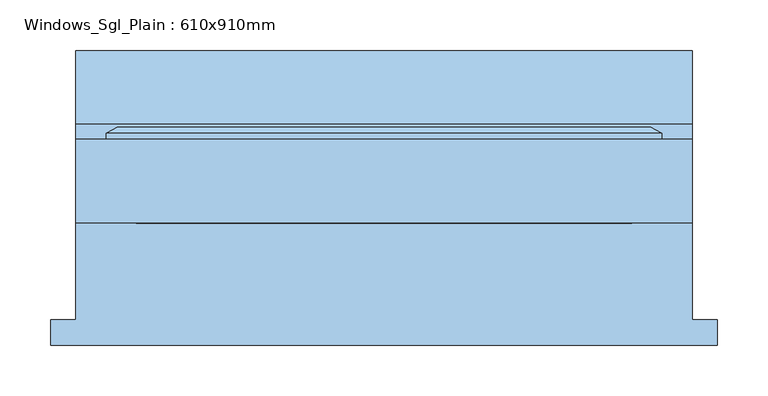
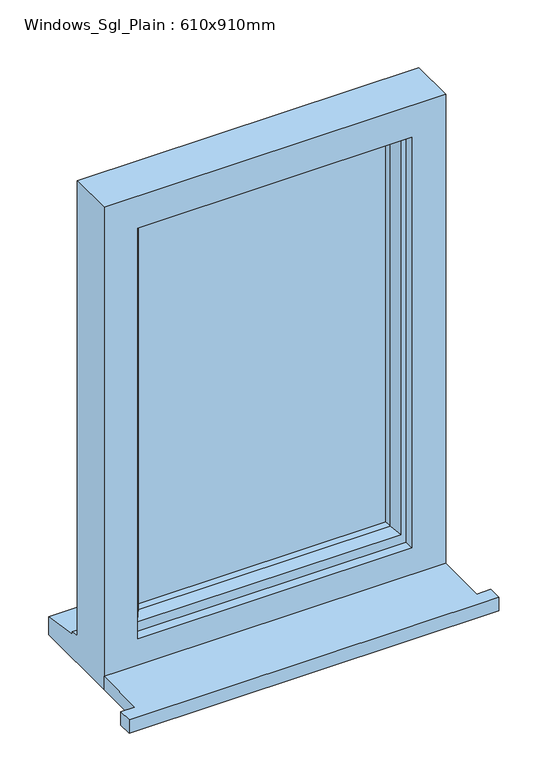
"""IFC4 building model written with IfcOpenShell, lengths in millimetres: window geometry, Windows_Sgl_Plain : 610x910mm."""

from ifc_helpers import new_model, si_unit, frame, origin, place, context, project, spatial, polyline, outline, extrude, faceted_brep, source, transform, mapped, element, save


def windows_sgl_plain_610x910mm_8d1346b0(model_context):
    return source(origin(), model_context, "Body", "SolidModel", [
        extrude(outline(polyline([(-329.8, -130.8434322), (-329.8, -105.8434322), (-304.8, -105.8434322), (-304.8, -10.2434322), (304.8, -10.2434322), (304.8, -105.8434322), (329.8, -105.8434322), (329.8, -130.8434322), (-329.8, -130.8434322)])), frame((0.0, 0.0, 1200.0), z_axis=(0.0, 0.0, 1.0), x_axis=(1.0, 0.0, 0.0)), (0.0, 0.0, 1.0), 25.0),
        faceted_brep([(-304.8, -10.2434322, 1200.0), (304.8, -10.2434322, 1200.0), (304.8, -10.2434322, 2110.0), (-304.8, -10.2434322, 2110.0), (-244.8, -10.2434322, 2050.0), (244.8, -10.2434322, 2050.0), (244.8, -10.2434322, 1275.0), (-244.8, -10.2434322, 1275.0), (-304.8, 72.7565678, 2110.0), (-304.8, 72.7565678, 1251.0), (-304.8, 87.7565678, 1249.68767), (-304.8, 87.7565678, 1244.7449676), (-304.8, 160.2565678, 1233.8088847), (-304.8, 160.2565678, 1200.0), (304.8, 72.7565678, 2110.0), (304.8, 72.7565678, 1251.0), (-264.8, 72.7565678, 2070.0), (-264.8, 72.7565678, 1263.0), (264.8, 72.7565678, 1263.0), (264.8, 72.7565678, 2070.0), (-264.8, 7.7565678, 2070.0), (-264.8, 7.7565678, 1263.0), (264.8, 7.7565678, 2070.0), (264.8, 7.7565678, 1263.0), (-244.8, 7.7565678, 2050.0), (-244.8, 7.7565678, 1275.0), (244.8, 7.7565678, 1275.0), (244.8, 7.7565678, 2050.0), (304.8, 160.2565678, 1200.0), (304.8, 160.2565678, 1233.8088847), (304.8, 87.7565678, 1244.7449676), (304.8, 87.7565678, 1249.68767)], [[[0, 1, 2, 3], [4, 5, 6, 7]], [[0, 3, 8, 9, 10, 11, 12, 13]], [[9, 8, 14, 15], [16, 17, 18, 19]], [[17, 16, 20, 21]], [[20, 22, 23, 21], [24, 25, 26, 27]], [[24, 4, 7, 25]], [[3, 2, 14, 8]], [[16, 19, 22, 20]], [[5, 4, 24, 27]], [[15, 14, 2, 1, 28, 29, 30, 31]], [[19, 18, 23, 22]], [[5, 27, 26, 6]], [[28, 1, 0, 13]], [[29, 28, 13, 12]], [[30, 29, 12, 11]], [[31, 30, 11, 10]], [[15, 31, 10, 9]], [[21, 23, 18, 17]], [[7, 6, 26, 25]]]),
        extrude(outline(polyline([(234.8, 36.7565678), (-234.8, 36.7565678), (-234.8, 60.7565678), (234.8, 60.7565678), (234.8, 36.7565678)])), frame((0.0, 0.0, 1293.0), z_axis=(0.0, 0.0, 1.0), x_axis=(1.0, 0.0, 0.0)), (0.0, 0.0, 1.0), 747.0),
        faceted_brep([(-274.8, 72.7565678, 2080.0), (-274.8, 78.5300705, 2080.0), (-274.8, 78.5300705, 1253.0), (-274.8, 72.7565678, 1253.0), (-264.8, 7.7565678, 2070.0), (-264.8, 72.7565678, 2070.0), (-264.8, 72.7565678, 1263.0), (-264.8, 7.7565678, 1263.0), (-224.8, 22.2494677, 2030.0), (-234.9480377, 7.7565678, 2040.1480377), (-234.9480377, 7.7565678, 1292.8519623), (-224.8, 22.2494677, 1303.0), (-224.8, 36.7565678, 2030.0), (-224.8, 36.7565678, 1303.0), (-234.8, 60.7565678, 2040.0), (-234.8, 36.7565678, 2040.0), (-234.8, 36.7565678, 1293.0), (-234.8, 60.7565678, 1293.0), (-224.8, 78.5300705, 2030.0), (-224.8, 60.7565678, 2030.0), (-224.8, 60.7565678, 1303.0), (-224.8, 78.5300705, 1303.0), (-242.2457548, 84.3035732, 2047.4457548), (-242.2457548, 84.3035732, 1285.5542452), (-264.0153903, 84.3035732, 2069.2153903), (-264.0153903, 84.3035732, 1263.7846097), (274.8, 78.5300705, 1253.0), (274.8, 72.7565678, 1253.0), (264.8, 72.7565678, 1263.0), (264.8, 7.7565678, 1263.0), (234.9480377, 7.7565678, 1292.8519623), (224.8, 22.2494677, 1303.0), (224.8, 36.7565678, 1303.0), (234.8, 36.7565678, 1293.0), (234.8, 60.7565678, 1293.0), (224.8, 60.7565678, 1303.0), (224.8, 78.5300705, 1303.0), (242.2457548, 84.3035732, 1285.5542452), (264.0153903, 84.3035732, 1263.7846097), (274.8, 78.5300705, 2080.0), (274.8, 72.7565678, 2080.0), (264.8, 72.7565678, 2070.0), (264.8, 7.7565678, 2070.0), (234.9480377, 7.7565678, 2040.1480377), (224.8, 22.2494677, 2030.0), (224.8, 36.7565678, 2030.0), (234.8, 36.7565678, 2040.0), (234.8, 60.7565678, 2040.0), (224.8, 60.7565678, 2030.0), (224.8, 78.5300705, 2030.0), (242.2457548, 84.3035732, 2047.4457548), (264.0153903, 84.3035732, 2069.2153903)], [[[0, 1, 2, 3]], [[4, 5, 6, 7]], [[8, 9, 10, 11]], [[12, 8, 11, 13]], [[14, 15, 16, 17]], [[18, 19, 20, 21]], [[22, 18, 21, 23]], [[1, 24, 25, 2]], [[3, 2, 26, 27]], [[7, 6, 28, 29]], [[11, 10, 30, 31]], [[13, 11, 31, 32]], [[17, 16, 33, 34]], [[21, 20, 35, 36]], [[23, 21, 36, 37]], [[2, 25, 38, 26]], [[27, 26, 39, 40]], [[29, 28, 41, 42]], [[31, 30, 43, 44]], [[32, 31, 44, 45]], [[34, 33, 46, 47]], [[36, 35, 48, 49]], [[37, 36, 49, 50]], [[26, 38, 51, 39]], [[40, 39, 1, 0]], [[3, 27, 40, 0], [5, 41, 28, 6]], [[42, 41, 5, 4]], [[7, 29, 42, 4], [9, 43, 30, 10]], [[44, 43, 9, 8]], [[45, 44, 8, 12]], [[15, 46, 33, 16], [13, 32, 45, 12]], [[47, 46, 15, 14]], [[17, 34, 47, 14], [19, 48, 35, 20]], [[49, 48, 19, 18]], [[50, 49, 18, 22]], [[24, 51, 38, 25], [23, 37, 50, 22]], [[39, 51, 24, 1]]]),
    ])


if __name__ == "__main__":
    model = new_model("IFC4")
    model_context = context("Model", 3, world=origin())
    ifc_project = project(units=[si_unit("LENGTHUNIT", "METRE", prefix="MILLI")], contexts=[model_context])
    site = spatial("IfcSite", under=ifc_project)
    building = spatial("IfcBuilding", under=site)
    placement = place(None, origin())
    windows_sgl_plain_610x910mm_shape = windows_sgl_plain_610x910mm_8d1346b0(model_context)
    element("IfcWindow", 1, ObjectType="Windows_Sgl_Plain : 610x910mm", at=placement, inside=building, context=model_context, shape_type="MappedRepresentation", body=[
        mapped(windows_sgl_plain_610x910mm_shape, transform((0.0, 0.0, 0.0), x_axis=(1.0, 0.0, 0.0), y_axis=(0.0, 1.0, 0.0), z_axis=(0.0, 0.0, 1.0))),
    ])
    save(model, "model.ifc")

# Revit data of these elements
# Type "Windows_Sgl_Plain : 610x910mm"
#   Type Mark = "44"
#   Operation = "SinglePanel"
#   Construction Type Id = "SGL"
#   Manufacturer = "Revit"
#   Keynote = "L10"
#   Analytic Construction = "Large single-glazed windows"
#   Wrap Layers (Ext) from Ext = 0' - 4.03543"
#   Wrap Layers (Int) from Ext = 0' - 6.98819"
#   Window Board Projection = 0' - 0.98425"
#   Window Board Extension = 0' - 0.98425"
#   Visual Light Transmittance = 0.9
#   Solar Heat Gain Coefficient = 0.86
#   Rough Width = 2' - 0"
#   Rough Height = 2' - 11.82677"
#   Height = 2' - 11.82677"
#   Width = 2' - 0"
#   Heat Transfer Coefficient (U) = 5.5617 W/(m²·K)
#   Glazing Thickness = 0' - 0.94488"
#   FrameOffset - External = 0' - 1.9685"
#   Frame Depth = 0' - 2.55906"
#   Default Head Height = 6' - 11.07087"
#   Cill Depth = 0' - 3.44488"
#   Cavity Closer Width = 0' - 1.9685"
#   Cavity Closer Offset from Ext = 0' - 4.03543"
#   Cavity Closer Depth = 0' - 3.34646"
#   Define Thermal Properties by = 1
#   Vis - Cavity Closers = yes
#   Define Thermal Properties by = 1
#   Material Trim = Window Frame
#   Material Glass = Glass
#   Material Frame = Window Frame
#   Wall Closure = (empty or 0)
# Element 1 (IfcWindow, "Windows_Sgl_Plain : 610x910mm")
#   Materials on its faces: "Window Frame", "Glass"
# Materials
#   "Window Frame": colour RGB 249 249 249, transparency 0, Keynote = "L10", Cost = 0
#   "Glass": class "Glass", colour RGB 0 128 192, transparency 0.9, Description = "Soda Lime Glass", Cost = 0
